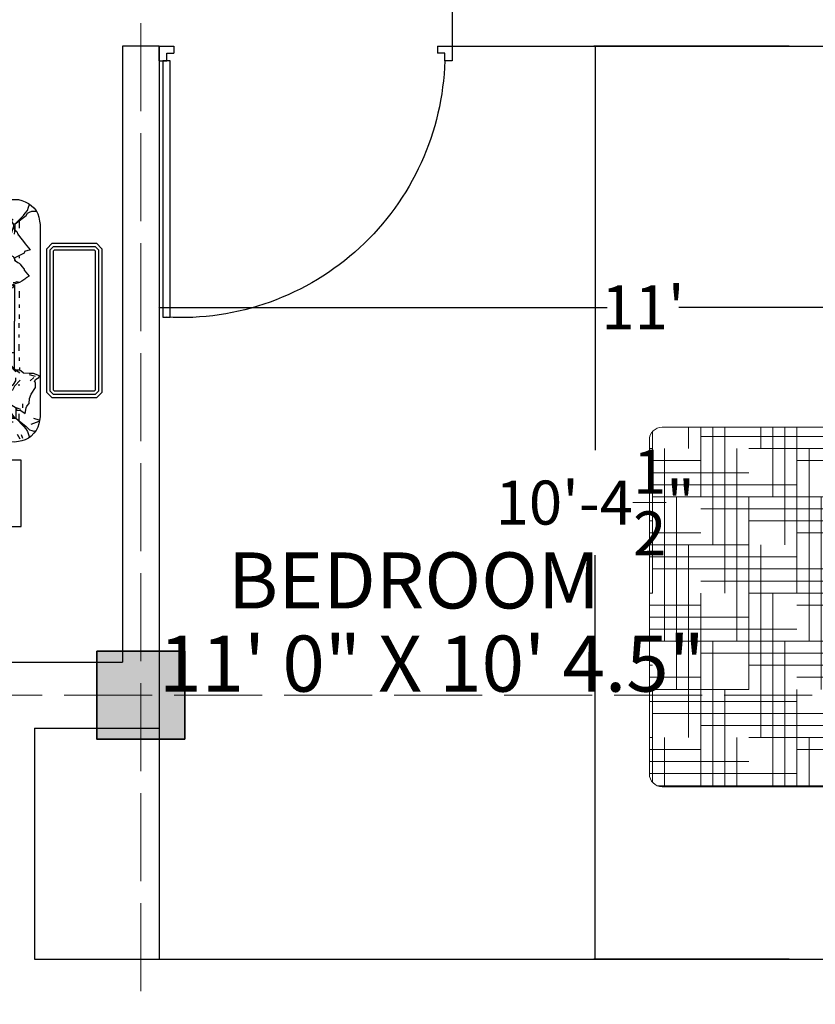
# Model space of a CAD drawing. Units: inches. Extents: x -113 to 5399, y -1393 to 3302.
# Tile 38 of 40: x 3504 to 3612, y 2903 to 3038. Entities that reach past the tile are written whole.
import ezdxf

# ---------------------------------------------------------------- set-up
doc = ezdxf.new("R2010")
doc.units = ezdxf.units.IN
doc.header["$MEASUREMENT"] = 0
doc.linetypes.add('ACAD_ISO02W100', pattern=[15, 12, -3])
doc.layers.add('24', color=7, linetype='Continuous')
for name, color, linetype, lineweight in [('A-ANNO-DIMS', 254, 'Continuous', 18), ('A-AREA-IDEN', 4, 'Continuous', 18), ('A-COLS', 7, 'Continuous', 35), ('doors', 2, 'Continuous', 25), ('furniture', 131, 'Continuous', 18), ('GRIDS', 7, 'ACAD_ISO02W100', 13), ('walls', 1, 'Continuous', 25)]:
    doc.layers.add(name, color=color, linetype=linetype, lineweight=lineweight)
doc.styles.get("Standard").update_dxf_attribs({"font": 'arial.ttf'})
doc.dimstyles.get("Standard").update_dxf_attribs({"dimtxt": 6, "dimasz": 0.18, "dimexe": 0.18, "dimexo": 0.0625, "dimgap": 0.09, "dimtad": 0, "dimtih": 1, "dimtoh": 1, "dimdec": 1, "dimzin": 0, "dimdsep": 46, "dimlunit": 4, "dimtxsty": 'Standard', "dimblk": 'ARCHTICK', "dimcen": 0.09, "dimadec": 0, "dimazin": 0, "dimtfac": 1, "dimtdec": 1, "dimtofl": 0, "dimtmove": 0, "dimatfit": 3, "dimfxl": 1, "dimtolj": 1, "dimtzin": 0, "dimarcsym": 0})

# ---------------------------------------------------------------- blocks, each defined once
blk = doc.blocks.new('*X4')
at = {"color": 0}
for p, q in [((4.3594, 18.5625), (4.3594, 18.6457)), ((4.5, 18), (4.5, 18.6457)), ((4.5469, 18.1875), (4.5469, 18.6457)), ((4.5938, 18.375), (4.5938, 18.6457)), ((4.6406, 18.5625), (4.6406, 18.6457)), ((4.7812, 18), (4.7812, 18.6457)), ((4.8281, 18.1875), (4.8281, 18.6457)), ((4.875, 18.375), (4.875, 18.6457)), ((4.9219, 18.5625), (4.9219, 18.6457)), ((5.0625, 18), (5.0625, 18.6457)), ((5.1094, 18.1875), (5.1094, 18.6457)), ((5.1562, 18.375), (5.1562, 18.6457)), ((5.2031, 18.5625), (5.2031, 18.6457)), ((5.3438, 18), (5.3438, 18.6457)), ((5.3906, 18.1875), (5.3906, 18.6457)), ((5.4375, 18.375), (5.4375, 18.6457)), ((5.4844, 18.5625), (5.4844, 18.6457)), ((4.6875, 18.6094), (5.4375, 18.6094)), ((5.625, 18), (5.625, 18.6287)), ((4.4531, 17.8169), (4.4531, 18.5625)), ((4.5, 18.5625), (5.25, 18.5625)), ((4.7344, 17.8125), (4.7344, 18.5625)), ((5.0156, 17.8125), (5.0156, 18.5625)), ((5.2969, 17.8125), (5.2969, 18.5625)), ((5.5781, 17.8125), (5.5781, 18.5625)), ((5.625, 18.5625), (5.6375, 18.5625)), ((4.3395, 18.5156), (5.0625, 18.5156)), ((5.4375, 18.5156), (5.6375, 18.5156)), ((4.3395, 18.4688), (4.875, 18.4688)), ((5.25, 18.4688), (5.6375, 18.4688)), ((4.3395, 18.4219), (4.6875, 18.4219)), ((5.0625, 18.4219), (5.6375, 18.4219)), ((4.3395, 18.375), (4.5, 18.375)), ((4.4062, 17.8169), (4.4062, 18.375)), ((4.6875, 17.8114), (4.6875, 18.375)), ((4.875, 18.375), (5.625, 18.375)), ((4.9688, 17.625), (4.9688, 18.375)), ((5.25, 17.625), (5.25, 18.375)), ((5.5312, 17.625), (5.5312, 18.375)), ((4.6875, 18.3281), (5.4375, 18.3281)), ((4.5, 18.2812), (5.25, 18.2812)), ((5.625, 18.2812), (5.6375, 18.2812)), ((4.3395, 18.2344), (5.0625, 18.2344)), ((5.4375, 18.2344), (5.6375, 18.2344)), ((4.3395, 18.1875), (4.875, 18.1875)), ((4.3594, 17.8169), (4.3594, 18.1875)), ((4.6406, 17.8169), (4.6406, 18.1875)), ((4.9219, 17.4375), (4.9219, 18.1875)), ((5.2031, 17.4375), (5.2031, 18.1875)), ((5.25, 18.1875), (5.6375, 18.1875)), ((5.4844, 17.4375), (5.4844, 18.1875)), ((4.3395, 18.1406), (4.6875, 18.1406)), ((5.0625, 18.1406), (5.6375, 18.1406)), ((4.3395, 18.0938), (4.5, 18.0938)), ((4.875, 18.0938), (5.625, 18.0938)), ((4.6875, 18.0469), (5.4375, 18.0469)), ((4.5, 18), (5.25, 18)), ((4.5938, 17.8169), (4.5938, 18)), ((4.875, 17.25), (4.875, 18)), ((5.1562, 17.25), (5.1562, 18)), ((5.4375, 17.25), (5.4375, 18)), ((5.625, 18), (5.6375, 18)), ((4.3395, 17.9531), (5.0625, 17.9531)), ((5.4375, 17.9531), (5.6375, 17.9531)), ((4.3395, 17.9062), (4.875, 17.9062)), ((5.25, 17.9062), (5.6375, 17.9062)), ((4.3395, 17.8594), (4.6875, 17.8594)), ((5.0625, 17.8594), (5.6375, 17.8594)), ((4.8281, 17.2457), (4.8281, 17.8125)), ((4.875, 17.8125), (5.625, 17.8125)), ((5.1094, 17.2457), (5.1094, 17.8125)), ((5.3906, 17.2457), (5.3906, 17.8125)), ((4.7421, 17.7656), (5.4375, 17.7656)), ((4.7548, 17.7188), (5.25, 17.7188)), ((5.625, 17.7188), (5.6375, 17.7188)), ((4.7548, 17.6719), (5.0625, 17.6719)), ((5.4375, 17.6719), (5.6375, 17.6719)), ((4.7548, 17.625), (4.875, 17.625)), ((4.7812, 17.2457), (4.7812, 17.625)), ((5.0625, 17.2457), (5.0625, 17.625)), ((5.25, 17.625), (5.6375, 17.625)), ((5.3438, 17.2457), (5.3438, 17.625)), ((5.625, 17.2627), (5.625, 17.625)), ((5.0625, 17.5781), (5.6375, 17.5781)), ((4.875, 17.5312), (5.625, 17.5312)), ((4.7548, 17.4844), (5.4375, 17.4844)), ((4.7548, 17.4375), (5.25, 17.4375)), ((5.0156, 17.2457), (5.0156, 17.4375)), ((5.2969, 17.2457), (5.2969, 17.4375)), ((5.5781, 17.2457), (5.5781, 17.4375)), ((5.625, 17.4375), (5.6375, 17.4375)), ((4.7548, 17.3906), (5.0625, 17.3906)), ((5.4375, 17.3906), (5.6375, 17.3906)), ((4.7548, 17.3438), (4.875, 17.3438)), ((5.25, 17.3438), (5.6375, 17.3438)), ((5.0625, 17.2969), (5.6375, 17.2969)), ((4.875, 17.25), (5.6077, 17.25)), ((4.9688, 17.2457), (4.9688, 17.25)), ((5.25, 17.2457), (5.25, 17.25)), ((5.5312, 17.2457), (5.5312, 17.25))]:
    blk.add_line(p, q, dxfattribs=at)
blk = doc.blocks.new('MAT-P01')
for p, q in [((0.0087, 0.8464), (0.2471, 0.8464)), ((0.3737, 0.8464), (1.6737, 0.8464)), ((1.7922, 0.8464), (2.0306, 0.8464)), ((-0.0213, 0.8164), (-0.0213, 0.5605)), ((0.2771, 0.8164), (0.2771, 0.5605)), ((0.3437, 0.8164), (0.3437, -0.0316)), ((1.7037, 0.8164), (1.7037, 0.5005)), ((1.7622, 0.8164), (1.7622, 0.5605)), ((2.0606, 0.8164), (2.0606, 0.5605)), ((0.0087, 0.5305), (0.2471, 0.5305)), ((0.9879, 0.5005), (1.0693, 0.5005)), ((1.6393, 0.5005), (1.7237, 0.5005)), ((1.7237, 0.5005), (1.7237, -0.8836)), ((1.7922, 0.5305), (2.0306, 0.5305)), ((0.8146, 0.423), (0.3237, -0.0509)), ((0.8949, 0.4293), (0.8949, 0.0491)), ((0.8949, 0.3643), (1.7237, 0.3643)), ((0.8949, 0.3643), (0.8949, 0.0491)), ((0.8949, 0.3643), (1.7237, 0.3643)), ((1.7237, 0.3643), (1.7237, -0.8836)), ((0.3237, -0.0509), (0.7949, -0.0509)), ((0.3237, -0.0509), (0.3237, -0.8836)), ((0.3737, -0.9336), (1.6737, -0.9336))]:
    blk.add_line(p, q)
for centre, radius, start, end in [((0.0087, 0.8164), 0.03, 90, 180), ((0.2471, 0.8164), 0.03, 0, 90), ((0.3737, 0.8164), 0.03, 90, 180), ((1.6737, 0.8164), 0.03, 0, 90), ((1.7922, 0.8164), 0.03, 90, 180), ((2.0306, 0.8164), 0.03, 0, 90), ((1.2251, 0.6034), 0.8138, 168.373, 191.627), ((0.7029, -1.1436), 1.9306, 81.8162, 98.1838), ((0.1806, 0.6034), 0.8138, 348.373, 11.627), ((1.8766, 0.6034), 0.8138, 168.373, 191.627), ((1.3543, -1.1436), 1.9306, 81.8162, 98.1838), ((0.8321, 0.6034), 0.8138, 348.373, 11.627), ((0.0087, 0.5605), 0.03, 180, 270), ((0.2471, 0.5605), 0.03, 270, 0), ((1.7922, 0.5605), 0.03, 180, 270), ((2.0306, 0.5605), 0.03, 270, 0), ((0.7029, 2.3504), 1.9306, 261.8162, 278.1838), ((1.3543, 2.3504), 1.9306, 261.8162, 278.1838), ((0.7949, 0.0491), 0.1, 270, 0), ((0.3737, -0.8836), 0.05, 180, 270), ((1.6737, -0.8836), 0.05, 270, 0)]:
    blk.add_arc(centre, radius, start, end)
at = {"rotation": 270}
blk.add_blockref('*X4', (-16.9221, 4.7038), dxfattribs=at)
blk = doc.blocks.new('DL13712')
at = {"layer": '24'}
for p, q in [((33, 28.5), (-34, 28.5)), ((33.5, -29.5), (-10, -29.5))]:
    blk.add_line(p, q, dxfattribs=at)
blk = doc.blocks.new('DL13976')
at = {"layer": '24'}
for p, q in [((-10.5, 16.5), (-7, 18.5)), ((-7, 18.5), (-3.5, 19.5)), ((-3.5, 19.5), (0.5, 20)), ((0.5, 20), (4.5, 19.5)), ((4.5, 19.5), (8, 18.5)), ((8, 18.5), (11.5, 16.5)), ((-18, 7.5), (-16, 11)), ((-16, 11), (-13.5, 14)), ((-13.5, 14), (-10.5, 16.5)), ((-4.5, 8), (-2.5, 9)), ((-2.5, 9), (0, 9.5)), ((0, 9.5), (2.5, 9.5)), ((0.5, -9.5), (0.5, 9.5)), ((2.5, 9.5), (5, 8.5)), ((11.5, 16.5), (14.5, 14)), ((14.5, 14), (17, 11)), ((17, 11), (19, 7.5)), ((-19.5, 0), (-19, 4)), ((-19, -4), (-19.5, 0)), ((-19, 4), (-18, 7.5)), ((-9, 2), (-8, 4.5)), ((-9, -0.5), (-9, 2)), ((-9, 0), (10, 0)), ((-8, 4.5), (-6.5, 6.5)), ((-6.5, 6.5), (-4.5, 8)), ((-5.5, 0), (6.5, 0)), ((0.5, -6), (0.5, 6)), ((5, 8.5), (7, 7)), ((7, 7), (8.5, 5)), ((8.5, 5), (9.5, 3)), ((9.5, 3), (10, 0.5)), ((10, 0.5), (10, -2)), ((19, 7.5), (20, 4)), ((20, 4), (20.5, 0)), ((20.5, 0), (20, -4)), ((-18, -7.5), (-19, -4)), ((-16, -11), (-18, -7.5)), ((-8.5, -3), (-9, -0.5)), ((-7.5, -5), (-8.5, -3)), ((-6, -7), (-7.5, -5)), ((-4, -8.5), (-6, -7)), ((-1.5, -9.5), (-4, -8.5)), ((5.5, -8), (3.5, -9)), ((7.5, -6.5), (5.5, -8)), ((9, -4.5), (7.5, -6.5)), ((10, -2), (9, -4.5)), ((19, -7.5), (17, -11)), ((20, -4), (19, -7.5)), ((-13.5, -14), (-16, -11)), ((-10.5, -16.5), (-13.5, -14)), ((-7, -18.5), (-10.5, -16.5)), ((1, -9.5), (-1.5, -9.5)), ((3.5, -9), (1, -9.5)), ((11.5, -16.5), (8, -18.5)), ((14.5, -14), (11.5, -16.5)), ((17, -11), (14.5, -14)), ((-3.5, -19.5), (-7, -18.5)), ((0.5, -20), (-3.5, -19.5)), ((4.5, -19.5), (0.5, -20)), ((8, -18.5), (4.5, -19.5))]:
    blk.add_line(p, q, dxfattribs=at)
blk = doc.blocks.new('DL13329')
at = {"layer": '24'}
for p, q in [((0, 0), (0, -60)), ((60, 0), (0, 0)), ((60, -60), (60, 0)), ((0, -60), (60, -60))]:
    blk.add_line(p, q, dxfattribs=at)
blk = doc.blocks.new('DL13303')
at = {"layer": '24'}
for p, q in [((-70, 20), (-65, 25)), ((-70, -20), (-70, 20)), ((-67, 19), (-64, 22)), ((-67, -19), (-67, 19)), ((-65, 25), (65, 25)), ((-64, 22), (64, 22)), ((-64, 18), (-63, 19)), ((-64, -18), (-64, 18)), ((-63, 19), (63, 19)), ((63, 19), (64, 18)), ((64, 22), (67, 19)), ((64, 18), (64, -18)), ((65, 25), (70, 20)), ((67, 19), (67, -19)), ((70, 20), (70, -20)), ((-65, -25), (-70, -20)), ((-64, -22), (-67, -19)), ((65, -25), (-65, -25)), ((-63, -19), (-64, -18)), ((64, -22), (-64, -22)), ((63, -19), (-63, -19)), ((64, -18), (63, -19)), ((67, -19), (64, -22)), ((70, -20), (65, -25))]:
    blk.add_line(p, q, dxfattribs=at)
blk = doc.blocks.new('DL12701')
at = {"layer": '24'}
for p, q in [((-93.5, 44.5), (-90, 45)), ((-90, 45), (-87, 45.5)), ((-87, 45.5), (0, 45.5)), ((0, 45.5), (87, 45.5)), ((50, 45), (48, 39.5)), ((51.5, 44.5), (50, 45)), ((87, 45.5), (90.5, 45)), ((90.5, 45), (93.5, 44.5)), ((-106, 35), (-104, 37.5)), ((-102.5, 35), (-105, 36)), ((-104, 37.5), (-102, 40)), ((-102, 40), (-99.5, 42)), ((-99.5, 42), (-96.5, 43.5)), ((-99, 40), (-99, 42)), ((-99, 38), (-99, 40)), ((-98, 36), (-99, 38)), ((-97, 34), (-98, 36)), ((-96.5, 43.5), (-93.5, 44.5)), ((-67.5, 33.5), (-64, 36.5)), ((-64, 36.5), (-62.5, 31.5)), ((48, 39.5), (48, 35.5)), ((50.5, 41.5), (49, 36)), ((53.5, 41.5), (51.5, 44.5)), ((51.5, 40), (54.5, 36.5)), ((55.5, 40.5), (53.5, 41.5)), ((56, 41.5), (55.5, 40.5)), ((60.5, 41.5), (56, 41.5)), ((66.5, 37.5), (60.5, 41.5)), ((70.5, 36), (66.5, 37.5)), ((75, 35.5), (70.5, 36)), ((88.5, 39.5), (90, 44.5)), ((91.5, 44.5), (94, 37)), ((93.5, 44.5), (96.5, 43.5)), ((96.5, 43.5), (99.5, 42)), ((97.5, 34.5), (99, 36)), ((99, 36), (99.5, 38)), ((99.5, 42), (102, 40)), ((100, 40), (99.5, 42)), ((99.5, 38), (100, 40)), ((102, 40), (104.5, 37.5)), ((103, 35), (106, 36)), ((104.5, 37.5), (106.5, 35)), ((-109.5, 26), (-108.5, 29)), ((-108.5, 29), (-107.5, 32)), ((-107.5, 32), (-106, 35)), ((-99.5, 34), (-102.5, 35)), ((-97, 32), (-99.5, 34)), ((-95, 33), (-97, 34)), ((-95, 30.5), (-97, 32)), ((-87.5, 23), (-95, 33)), ((-87.5, 23), (-95, 30.5)), ((-78, 25.5), (-76, 27)), ((-76, 27), (-71.5, 30.5)), ((-71.5, 30.5), (-69.5, 32)), ((-69.5, 32), (-67.5, 33.5)), ((-62.5, 31.5), (-61, 31)), ((-61, 31), (-59.5, 28)), ((-59.5, 28), (-57.5, 24.5)), ((-52, 26.5), (-51, 27.5)), ((-51, 27.5), (-49, 29)), ((-49, 29), (-46.5, 31)), ((-46.5, 31), (-45.5, 31)), ((-45.5, 31), (-40, 35.5)), ((-40, 35.5), (-38.5, 33)), ((-38.5, 33), (-38, 32.5)), ((-38, 32.5), (-35.5, 29)), ((-35.5, 29), (-34.5, 27)), ((-34.5, 27), (-35, 24.5)), ((-34.5, 27), (-33.5, 24)), ((42.5, 27), (45, 27)), ((45.5, 28), (45, 27)), ((45, 27), (45, 23.5)), ((47.5, 30.5), (45.5, 28)), ((46.5, 26), (47.5, 27)), ((48, 35.5), (47.5, 30.5)), ((54, 27.5), (59.5, 22.5)), ((77.5, 33.5), (75, 35.5)), ((79, 30), (75.5, 30)), ((79, 33), (77.5, 33.5)), ((84, 32), (79, 33)), ((80.5, 28), (79, 24)), ((81, 24.5), (81.5, 28)), ((81.5, 28), (84, 32)), ((88.5, 23.5), (96, 33)), ((88.5, 23.5), (95.5, 30.5)), ((95.5, 30.5), (98, 32.5)), ((96, 33), (97.5, 34.5)), ((98, 32.5), (100.5, 34)), ((100.5, 34), (103, 35)), ((103, 28.5), (106.5, 29.5)), ((107.5, 27.5), (103, 25)), ((106.5, 35), (108, 32)), ((108, 32), (109, 29)), ((109, 29), (109.5, 26)), ((-109.5, 22.5), (-109.5, 26)), ((-109.5, -26.5), (-109.5, 22.5)), ((-95, 18.5), (-92, 19.5)), ((-95, 18), (-95, 18.5)), ((-94, 16.5), (-95, 18)), ((-92, 19.5), (-89, 20)), ((-91, 21), (-91, 19.5)), ((-89.5, 26.5), (-83.5, 26.5)), ((-89, 20), (-87.5, 21)), ((-87.5, 21), (-87.5, 23)), ((-81.5, 23), (-87.5, 23)), ((-87.5, 21), (-85, 21.5)), ((-85, 21.5), (-82, 22.5)), ((-85, 21.5), (-80.5, 20)), ((-82, 22.5), (-80.5, 24.5)), ((-82, 22.5), (-80.5, 22.5)), ((-80.5, 24.5), (-78, 25.5)), ((-80.5, 24.5), (-80.5, 23.5)), ((-80.5, 22.5), (-78, 22)), ((-80.5, 20), (-79.5, 20)), ((-77, 25.5), (-77, 25.5)), ((-60.5, 17.5), (-59, 19.5)), ((-59, 19.5), (-58.5, 19.5)), ((-58.5, 19.5), (-58, 21)), ((-58, 26.5), (-56.5, 26.5)), ((-58, 21), (-54.5, 23)), ((-57.5, 24.5), (-56.5, 22)), ((-56.5, 22.5), (-54.5, 22.5)), ((-54.5, 22.5), (-52.5, 25.5)), ((-54.5, 23), (-54.5, 22.5)), ((-54, 22.5), (-54, 22.5)), ((-52.5, 25.5), (-52, 26.5)), ((-35, 24.5), (-34.5, 23)), ((-34.5, 23), (-34, 21)), ((-33.5, 24), (-33, 22)), ((-30, 21), (-33, 22)), ((-33, 22), (-31.5, 19.5)), ((-32, 22.5), (0.5, 22.5)), ((-31.5, 19.5), (-31, 18)), ((-29.5, 19.5), (-30, 21)), ((-28.5, 16.5), (-29.5, 19.5)), ((-26.5, 26.5), (-20.5, 26.5)), ((-14.5, 26.5), (-11.5, 26.5)), ((-5.5, 26.5), (-1.5, 26.5)), ((44, 22.5), (0.5, 22.5)), ((6.5, 26.5), (2.5, 26.5)), ((15.5, 26.5), (12.5, 26.5)), ((27.5, 26.5), (21.5, 26.5)), ((33.5, 26.5), (36.5, 26.5)), ((40.5, 18.5), (38, 14.5)), ((41.5, 20), (40.5, 18.5)), ((43.5, 22), (41.5, 20)), ((43.5, 20.5), (41.5, 20)), ((45, 23.5), (43.5, 22)), ((45, 22), (43.5, 20.5)), ((45, 23.5), (46.5, 26)), ((46.5, 23.5), (45, 22)), ((54.5, 23.5), (52, 23.5)), ((58, 21.5), (54.5, 23.5)), ((59, 26.5), (57.5, 26.5)), ((59.5, 19), (58, 21.5)), ((59.5, 22.5), (63, 20.5)), ((64, 17.5), (59.5, 19)), ((63, 20.5), (64, 17.5)), ((76, 19), (79, 24)), ((76, 16), (76, 19)), ((79, 24), (81, 24.5)), ((79, 23.5), (88.5, 23.5)), ((82.5, 18.5), (88, 22.5)), ((90.5, 26.5), (84.5, 26.5)), ((85, 16), (88, 22.5)), ((88.5, 8), (88.5, 23.5)), ((92, 21), (92, 15)), ((109.5, 26), (110, 22.5)), ((110, 22.5), (109.5, -26.5)), ((-92.5, 14), (-94, 16.5)), ((-92, 13.5), (-92.5, 14)), ((-91.5, 12.5), (-92, 13.5)), ((-89.5, 11), (-91.5, 12.5)), ((-91, 9), (-91, 6)), ((-89, 9), (-89.5, 11)), ((-89, 8.5), (-89, 9)), ((-74, 14.5), (-77.5, 15)), ((-70.5, 13.5), (-74, 14.5)), ((-74, 14.5), (-71, 10)), ((-71, 10), (-68, 8.5)), ((-67.5, 10.5), (-70.5, 13.5)), ((-68, 12), (-67.5, 12.5)), ((-65, 9), (-68, 12)), ((-67.5, 12.5), (-66.5, 13.5)), ((-61.5, 5.5), (-67.5, 10.5)), ((-66.5, 13.5), (-64.5, 15.5)), ((-63, 9), (-65, 9)), ((-64.5, 15.5), (-63.5, 15.5)), ((-63.5, 15.5), (-62.5, 16.5)), ((-62, 6.5), (-63, 9)), ((-62.5, 16.5), (-60.5, 17.5)), ((-46.5, 7.5), (-42.5, 10.5)), ((-40, 9), (-43.5, 7.5)), ((-42.5, 10.5), (-40, 11.5)), ((-40, 11.5), (-37, 13.5)), ((-32.5, 11.5), (-40, 9)), ((-37, 13.5), (-36, 14.5)), ((-24.5, 13.5), (-28.5, 16.5)), ((-21, 11), (-24.5, 13.5)), ((-19, 8.5), (-22.5, 11.5)), ((-17, 8), (-21, 11)), ((38, 14), (37.5, 11)), ((37.5, 11), (43.5, 8.5)), ((38, 14.5), (38, 14)), ((64, 17.5), (66.5, 14.5)), ((70.5, 13.5), (70.5, 14.5)), ((73, 8.5), (70.5, 13.5)), ((73, 13), (72.5, 15)), ((73, 12.5), (75, 14.5)), ((73, 12.5), (73, 13)), ((73, 8.5), (73, 12.5)), ((76, 12.5), (74, 14)), ((75, 14.5), (76, 16)), ((75.5, 16), (76, 16.5)), ((80, 11), (76, 12.5)), ((80.5, 9), (79, 9)), ((80.5, 10.5), (80, 11)), ((83, 8.5), (80.5, 10.5)), ((83, 8.5), (80.5, 9)), ((92, 9), (92, 6)), ((-91, 0.5), (-91, -5.5)), ((-89, 6), (-89, 8.5)), ((-86.5, 3.5), (-89, 6)), ((-87, 3.5), (-87, -26.5)), ((-86, 3.5), (-86.5, 3.5)), ((-85.5, 0.5), (-86, 3.5)), ((-85.5, 0), (-85.5, 0.5)), ((-84.5, -2), (-85.5, 0)), ((-68, 8.5), (-66.5, 5.5)), ((-66.5, 5.5), (-66, 4)), ((-62.5, 0), (-63.5, -1)), ((-60, 6), (-62, 6.5)), ((-61, -2), (-58.5, 0.5)), ((-57.5, 3.5), (-60, 6)), ((-60, 6), (-55, 5.5)), ((-58.5, 0.5), (-55.5, 2)), ((-56.5, 3.5), (-57.5, 3.5)), ((-57.5, 3.5), (-56, 1.5)), ((-54, 3), (-56.5, 3.5)), ((-56, 1.5), (-55, 0)), ((-55, 5.5), (-54, 5)), ((-55, 0), (-52.5, -2.5)), ((-46.5, 7.5), (-50.5, 8.5)), ((-43.5, 7.5), (-46.5, 7.5)), ((-31.5, -3), (-25.5, 0)), ((-25.5, 0), (-23, 3.5)), ((-20.5, 7.5), (-25, 7)), ((-23, 5.5), (-21.5, 6)), ((-23, 3.5), (-23, 5.5)), ((-21.5, 6), (-18, 6)), ((-18, 6), (-17, 8)), ((43.5, 8.5), (44, 8)), ((44, 8), (47, 6.5)), ((47, 6.5), (49.5, 5.5)), ((49.5, 5.5), (51, 5)), ((51, 5), (52.5, 5)), ((52, -2.5), (55, 1)), ((52.5, 5), (55.5, 5)), ((55, 1), (57.5, 3)), ((55.5, 5), (55.5, 5)), ((55.5, 5), (59, 2.5)), ((59, 2.5), (60, 3.5)), ((60, 3.5), (60, 2.5)), ((60, 2.5), (63, 2)), ((63, 2), (64, 1)), ((64, 1), (66, 0.5)), ((66, 0.5), (66.5, 0)), ((66.5, 0), (69, -0.5)), ((71.5, -1), (72.5, 2.5)), ((72, 5), (73, 6.5)), ((73, 5.5), (72, -1)), ((72.5, 2.5), (72, 5)), ((73, 6.5), (73, 8.5)), ((74.5, -0.5), (76, 1.5)), ((76, 1.5), (76.5, 3)), ((84, 6.5), (81.5, 6.5)), ((85, 8), (83, 8.5)), ((85.5, 6.5), (84, 6.5)), ((88, 7.5), (85, 8)), ((88, 7.5), (85.5, 6.5)), ((90, 6.5), (88, 7.5)), ((94, 5), (90, 6.5)), ((95, 4.5), (94, 5)), ((94, -3), (97.5, 3)), ((97.5, 3), (95, 4.5)), ((-83, -4), (-84.5, -2)), ((-80.5, -6.5), (-83, -4)), ((-80.5, -7), (-80.5, -6.5)), ((-77.5, -13), (-80.5, -7)), ((-70.5, -8.5), (-73.5, -11)), ((-68.5, -7), (-70.5, -8.5)), ((-68.5, -4.5), (-67, -3)), ((-66.5, -4.5), (-68.5, -7)), ((-68.5, -7), (-68.5, -4.5)), ((-67, -3), (-66, -1)), ((-65.5, -3), (-66.5, -4.5)), ((-63.5, -1), (-65.5, -3)), ((-65.5, -3), (-62.5, -2.5)), ((-62.5, -2.5), (-61, -2)), ((-54, -0.5), (-53.5, -0.5)), ((-52.5, -2.5), (-49.5, -7.5)), ((-49.5, -7.5), (-49.5, -9)), ((-45.5, -11), (-48.5, -7.5)), ((-43, -10), (-41.5, -7)), ((-38, -9), (-35, -6.5)), ((-35, -6.5), (-31.5, -3)), ((48, -10), (51.5, -6)), ((51.5, -5.5), (52, -2.5)), ((51.5, -6), (51.5, -5.5)), ((52, -8), (55.5, -5.5)), ((69, -0.5), (70.5, -1)), ((70.5, -1), (71.5, -1)), ((72, -1), (70.5, -5)), ((70.5, -5), (72.5, -8)), ((72.5, -8), (74.5, -3.5)), ((72.5, -8), (73, -12.5)), ((74.5, -3.5), (74.5, -0.5)), ((91, -10), (92, -8.5)), ((92, -8.5), (93, -7)), ((93, -7), (93.5, -4)), ((93.5, -4), (94, -3)), ((-91, -14), (-91, -11)), ((-74.5, -11.5), (-77.5, -13)), ((-73.5, -11), (-74.5, -11.5)), ((-49.5, -9), (-47, -11.5)), ((-47, -11.5), (-45, -15.5)), ((-45, -15.5), (-42, -11.5)), ((-42, -11.5), (-41, -11)), ((-41, -11), (-38, -9)), ((52, -12), (48, -10)), ((52, -10), (56.5, -12.5)), ((55, -13), (52, -12)), ((56.5, -13), (55, -13)), ((62.5, -16), (56.5, -13)), ((64.5, -17), (62.5, -16)), ((64, -16.5), (64, -16.5)), ((66.5, -18), (64.5, -17)), ((67.5, -15.5), (68.5, -18)), ((70, -16.5), (69.5, -15.5)), ((72, -21), (70, -16.5)), ((85, -17.5), (87, -16.5)), ((85, -18), (85, -17.5)), ((87, -16.5), (88, -13)), ((87.5, -12.5), (89.5, -11)), ((88, -13), (87.5, -12.5)), ((87.5, -26.5), (87.5, -14.5)), ((89.5, -11), (91, -10)), ((92, -14), (92, -11)), ((-109.5, -28), (-109.5, -26.5)), ((-109.5, -26.5), (-109.5, -29.5)), ((-106, -26), (-104.5, -26)), ((-102.5, -26), (-100.5, -26)), ((-98.5, -26), (-96, -26)), ((-94.5, -26), (-92.5, -26)), ((-91, -26), (-91, -20)), ((-87, -26.5), (-87, -28)), ((69, -18.5), (66.5, -18)), ((68.5, -18), (69, -18.5)), ((69, -18.5), (72, -21)), ((72, -21), (73, -22.5)), ((73, -22.5), (74.5, -23.5)), ((74.5, -23.5), (76, -26)), ((76, -26), (79, -28)), ((79.5, -27.5), (80, -26)), ((80, -26), (82.5, -23.5)), ((82.5, -21.5), (83.5, -20)), ((82.5, -22.5), (82.5, -21.5)), ((82.5, -23.5), (82.5, -22.5)), ((83.5, -20), (85, -18)), ((87.5, -28), (87.5, -26.5)), ((92, -26), (92, -20)), ((95.5, -26), (93.5, -26)), ((99.5, -26), (97, -26)), ((103.5, -26), (101.5, -26)), ((107, -26), (105.5, -26)), ((110, -29.5), (109.5, -26.5)), ((109.5, -26.5), (109.5, -28)), ((-109, -29), (-109.5, -28)), ((-109.5, -29.5), (-109, -32.5)), ((-108.5, -30), (-109, -29)), ((-109, -32.5), (-108, -35)), ((-108, -31), (-108.5, -30)), ((-106.5, -31.5), (-108, -31)), ((-108, -35), (-107, -37.5)), ((-105.5, -31.5), (-106.5, -31.5)), ((-104.5, -31.5), (-105.5, -31.5)), ((-92, -31.5), (-104.5, -31.5)), ((-91, -31.5), (-92, -31.5)), ((-90, -31.5), (-91, -31.5)), ((-90.5, -27.5), (-88, -28)), ((-90.5, -28), (-90, -29)), ((-89, -30.5), (-90, -31.5)), ((-88, -30), (-89, -30.5)), ((-87.5, -29), (-88, -30)), ((-87, -28), (-87.5, -29)), ((79, -28), (79.5, -27.5)), ((87.5, -29), (87.5, -28)), ((88, -30), (87.5, -29)), ((89, -30.5), (88, -30)), ((91.5, -27.5), (89, -28)), ((90, -31.5), (89, -30.5)), ((91, -31.5), (90, -31.5)), ((91.5, -28), (91, -29)), ((92.5, -31.5), (91, -31.5)), ((104.5, -31.5), (92.5, -31.5)), ((106, -31.5), (104.5, -31.5)), ((107, -31.5), (106, -31.5)), ((108, -31), (107, -31.5)), ((107, -37.5), (108.5, -35)), ((109, -30), (108, -31)), ((108.5, -35), (109.5, -32.5)), ((109.5, -29), (109, -30)), ((109.5, -28), (109.5, -29)), ((109.5, -32.5), (110, -29.5)), ((-107, -37.5), (-105, -39.5)), ((-105, -39.5), (-102.5, -41.5)), ((-102.5, -41.5), (-100, -43)), ((-100.5, -37), (-100.5, -40.5)), ((-100, -43), (-97.5, -44)), ((-94.5, -39.5), (-98.5, -42.5)), ((-97.5, -44), (-94.5, -44.5)), ((-94.5, -44.5), (0, -44.5)), ((-67, -37), (-64.5, -40.5)), ((-45, -37.5), (-49.5, -41)), ((-27.5, -37.5), (-29.5, -42.5)), ((0, -44.5), (95, -44.5)), ((28.5, -37.5), (30.5, -42.5)), ((46, -37.5), (50.5, -41)), ((68, -37), (65.5, -40.5)), ((95, -44.5), (97.5, -44)), ((95.5, -39.5), (99.5, -42.5)), ((97.5, -44), (100.5, -43)), ((100.5, -43), (103, -41.5)), ((101.5, -37), (101.5, -40.5)), ((103, -41.5), (105, -39.5)), ((105, -39.5), (107, -37.5))]:
    blk.add_line(p, q, dxfattribs=at)
blk = doc.blocks.new('DL13707')
at = {"layer": '24'}
for p, q in [((0, -33.5), (0, 33.5)), ((-58.5, -33.5), (-58.5, 21.5)), ((58.5, -33.5), (58.5, 2))]:
    blk.add_line(p, q, dxfattribs=at)
blk = doc.blocks.new('DL13651')
at = {"layer": '24'}
for p, q in [((-50.5, 25), (-50, 27)), ((-50, 27), (-49, 28.5)), ((-49, 28.5), (-47.5, 29.5)), ((-47.5, 29.5), (-45.5, 30)), ((-45.5, 30), (44.5, 30)), ((44.5, 30), (46.5, 29.5)), ((46.5, 29.5), (48, 28.5)), ((48, 28.5), (49, 27)), ((49, 27), (49.5, 25)), ((-50.5, -25), (-50.5, 25)), ((-45.5, 24.5), (-45.5, 25)), ((-45.5, 25), (-45, 25)), ((-45.5, -24.5), (-45.5, 24.5)), ((-45, 25), (44, 25)), ((-45, 22), (44, 22)), ((-42.5, 22), (-45, 22)), ((-42.5, -24.5), (-42.5, 24.5)), ((-42.5, 24.5), (-42.5, 22)), ((41.5, 22), (41.5, 24.5)), ((41.5, 24.5), (41.5, -24.5)), ((44, 22), (41.5, 22)), ((44, 25), (44.5, 25)), ((44.5, 25), (44.5, 24.5)), ((44.5, 24.5), (44.5, -24.5)), ((49.5, 25), (49.5, -25)), ((-50, -27), (-50.5, -25)), ((-45.5, -25), (-45.5, -24.5)), ((-45, -25), (-45.5, -25)), ((44, -22), (-45, -22)), ((-45, -22), (-42.5, -22)), ((44, -25), (-45, -25)), ((-42.5, -22), (-42.5, -24.5)), ((41.5, -24.5), (41.5, -22)), ((41.5, -22), (44, -22)), ((44.5, -25), (44, -25)), ((44.5, -24.5), (44.5, -25)), ((49.5, -25), (49, -27)), ((-49, -28.5), (-50, -27)), ((-47.5, -29.5), (-49, -28.5)), ((-45.5, -30), (-47.5, -29.5)), ((44.5, -30), (-45.5, -30)), ((46.5, -29.5), (44.5, -30)), ((48, -28.5), (46.5, -29.5)), ((49, -27), (48, -28.5))]:
    blk.add_line(p, q, dxfattribs=at)
blk = doc.blocks.new('DL12263')
at = {"layer": '24'}
for p, q in [((-112.5, 44.5), (-109, 45)), ((-109, 45), (-106, 45.5)), ((-106, 45.5), (-19, 45.5)), ((-19, 45.5), (106.5, 45.5)), ((69.5, 45), (67.5, 39.5)), ((71, 44.5), (69.5, 45)), ((106.5, 45.5), (110, 45)), ((110, 45), (113, 44.5)), ((-125, 35), (-123, 37.5)), ((-121.5, 35), (-124, 36)), ((-123, 37.5), (-121, 40)), ((-121, 40), (-118.5, 42)), ((-118.5, 42), (-115.5, 43.5)), ((-118, 40), (-118, 42)), ((-118, 38), (-118, 40)), ((-117, 36), (-118, 38)), ((-116, 34), (-117, 36)), ((-115.5, 43.5), (-112.5, 44.5)), ((-86.5, 33.5), (-83, 36.5)), ((-83, 36.5), (-81.5, 31.5)), ((67.5, 39.5), (67.5, 35.5)), ((70, 41.5), (68.5, 36)), ((73, 41.5), (71, 44.5)), ((71, 40), (74, 36.5)), ((75, 40.5), (73, 41.5)), ((75.5, 41.5), (75, 40.5)), ((80, 41.5), (75.5, 41.5)), ((86, 37.5), (80, 41.5)), ((90, 36), (86, 37.5)), ((94.5, 35.5), (90, 36)), ((108, 39.5), (109.5, 44.5)), ((111, 44.5), (113.5, 37)), ((113, 44.5), (116, 43.5)), ((116, 43.5), (119, 42)), ((117, 34.5), (118.5, 36)), ((118.5, 36), (119, 38)), ((119, 42), (121.5, 40)), ((119.5, 40), (119, 42)), ((119, 38), (119.5, 40)), ((121.5, 40), (124, 37.5)), ((122.5, 35), (125.5, 36)), ((124, 37.5), (126, 35)), ((-128.5, 26), (-127.5, 29)), ((-127.5, 29), (-126.5, 32)), ((-126.5, 32), (-125, 35)), ((-118.5, 34), (-121.5, 35)), ((-116, 32), (-118.5, 34)), ((-114, 33), (-116, 34)), ((-114, 30.5), (-116, 32)), ((-106.5, 23), (-114, 33)), ((-106.5, 23), (-114, 30.5)), ((-97, 25.5), (-95, 27)), ((-95, 27), (-90.5, 30.5)), ((-90.5, 30.5), (-88.5, 32)), ((-88.5, 32), (-86.5, 33.5)), ((-81.5, 31.5), (-80, 31)), ((-80, 31), (-78.5, 28)), ((-78.5, 28), (-76.5, 24.5)), ((-71, 26.5), (-70, 27.5)), ((-70, 27.5), (-68, 29)), ((-68, 29), (-65.5, 31)), ((-65.5, 31), (-64.5, 31)), ((-64.5, 31), (-59, 35.5)), ((-59, 35.5), (-57.5, 33)), ((-57.5, 33), (-57, 32.5)), ((-57, 32.5), (-54.5, 29)), ((-54.5, 29), (-53.5, 27)), ((-53.5, 27), (-54, 24.5)), ((-53.5, 27), (-52.5, 24)), ((62, 27), (64.5, 27)), ((65, 28), (64.5, 27)), ((64.5, 27), (64.5, 23.5)), ((67, 30.5), (65, 28)), ((66, 26), (67, 27)), ((67.5, 35.5), (67, 30.5)), ((73.5, 27.5), (79, 22.5)), ((97, 33.5), (94.5, 35.5)), ((98.5, 30), (95, 30)), ((98.5, 33), (97, 33.5)), ((103.5, 32), (98.5, 33)), ((100, 28), (98.5, 24)), ((100.5, 24.5), (101, 28)), ((101, 28), (103.5, 32)), ((108, 23.5), (115.5, 33)), ((108, 23.5), (115, 30.5)), ((115, 30.5), (117.5, 32.5)), ((115.5, 33), (117, 34.5)), ((117.5, 32.5), (120, 34)), ((120, 34), (122.5, 35)), ((122.5, 28.5), (126, 29.5)), ((127, 27.5), (122.5, 25)), ((126, 35), (127.5, 32)), ((127.5, 32), (128.5, 29)), ((128.5, 29), (129, 26)), ((-128.5, 22.5), (-128.5, 26)), ((-128.5, -26.5), (-128.5, 22.5)), ((-114, 18.5), (-111, 19.5)), ((-114, 18), (-114, 18.5)), ((-113, 16.5), (-114, 18)), ((-111, 19.5), (-108, 20)), ((-110, 21), (-110, 19.5)), ((-108.5, 26.5), (-102.5, 26.5)), ((-108, 20), (-106.5, 21)), ((-106.5, 21), (-106.5, 23)), ((-100.5, 23), (-106.5, 23)), ((-106.5, 21), (-104, 21.5)), ((-104, 21.5), (-101, 22.5)), ((-104, 21.5), (-99.5, 20)), ((-101, 22.5), (-99.5, 24.5)), ((-101, 22.5), (-99.5, 22.5)), ((-99.5, 24.5), (-97, 25.5)), ((-99.5, 24.5), (-99.5, 23.5)), ((-99.5, 22.5), (-97, 22)), ((-99.5, 20), (-98.5, 20)), ((-96, 25.5), (-96, 25.5)), ((-79.5, 17.5), (-78, 19.5)), ((-78, 19.5), (-77.5, 19.5)), ((-77.5, 19.5), (-77, 21)), ((-77, 26.5), (-75.5, 26.5)), ((-77, 21), (-73.5, 23)), ((-76.5, 24.5), (-75.5, 22)), ((-75.5, 22.5), (-73.5, 22.5)), ((-73.5, 22.5), (-71.5, 25.5)), ((-73.5, 23), (-73.5, 22.5)), ((-73, 22.5), (-73, 22.5)), ((-71.5, 25.5), (-71, 26.5)), ((-54, 24.5), (-53.5, 23)), ((-53.5, 23), (-53, 21)), ((-52.5, 24), (-52, 22)), ((-49, 21), (-52, 22)), ((-52, 22), (-50.5, 19.5)), ((-51, 22.5), (-18.5, 22.5)), ((-50.5, 19.5), (-50, 18)), ((-48.5, 19.5), (-49, 21)), ((-47.5, 16.5), (-48.5, 19.5)), ((-45.5, 26.5), (-39.5, 26.5)), ((-33.5, 26.5), (-30.5, 26.5)), ((-24.5, 26.5), (-20.5, 26.5)), ((63.5, 22.5), (-18.5, 22.5)), ((-12.5, 26.5), (-16.5, 26.5)), ((35, 26.5), (-6.5, 26.5)), ((47, 26.5), (41, 26.5)), ((53, 26.5), (56, 26.5)), ((60, 18.5), (57.5, 14.5)), ((61, 20), (60, 18.5)), ((63, 22), (61, 20)), ((63, 20.5), (61, 20)), ((64.5, 23.5), (63, 22)), ((64.5, 22), (63, 20.5)), ((64.5, 23.5), (66, 26)), ((66, 23.5), (64.5, 22)), ((74, 23.5), (71.5, 23.5)), ((77.5, 21.5), (74, 23.5)), ((78.5, 26.5), (77, 26.5)), ((79, 19), (77.5, 21.5)), ((79, 22.5), (82.5, 20.5)), ((83.5, 17.5), (79, 19)), ((82.5, 20.5), (83.5, 17.5)), ((95.5, 19), (98.5, 24)), ((95.5, 16), (95.5, 19)), ((98.5, 24), (100.5, 24.5)), ((98.5, 23.5), (108, 23.5)), ((102, 18.5), (107.5, 22.5)), ((110, 26.5), (104, 26.5)), ((104.5, 16), (107.5, 22.5)), ((108, 8), (108, 23.5)), ((111.5, 21), (111.5, 15)), ((129, 26), (129.5, 22.5)), ((129.5, 22.5), (129, -26.5)), ((-111.5, 14), (-113, 16.5)), ((-111, 13.5), (-111.5, 14)), ((-110.5, 12.5), (-111, 13.5)), ((-108.5, 11), (-110.5, 12.5)), ((-110, 9), (-110, 6)), ((-108, 9), (-108.5, 11)), ((-108, 8.5), (-108, 9)), ((-93, 14.5), (-96.5, 15)), ((-89.5, 13.5), (-93, 14.5)), ((-93, 14.5), (-90, 10)), ((-90, 10), (-87, 8.5)), ((-86.5, 10.5), (-89.5, 13.5)), ((-87, 12), (-86.5, 12.5)), ((-84, 9), (-87, 12)), ((-86.5, 12.5), (-85.5, 13.5)), ((-80.5, 5.5), (-86.5, 10.5)), ((-85.5, 13.5), (-83.5, 15.5)), ((-82, 9), (-84, 9)), ((-83.5, 15.5), (-82.5, 15.5)), ((-82.5, 15.5), (-81.5, 16.5)), ((-81, 6.5), (-82, 9)), ((-81.5, 16.5), (-79.5, 17.5)), ((-65.5, 7.5), (-61.5, 10.5)), ((-59, 9), (-62.5, 7.5)), ((-61.5, 10.5), (-59, 11.5)), ((-59, 11.5), (-56, 13.5)), ((-51.5, 11.5), (-59, 9)), ((-56, 13.5), (-55, 14.5)), ((-43.5, 13.5), (-47.5, 16.5)), ((-40, 11), (-43.5, 13.5)), ((-38, 8.5), (-41.5, 11.5)), ((-36, 8), (-40, 11)), ((57.5, 14), (57, 11)), ((57, 11), (63, 8.5)), ((57.5, 14.5), (57.5, 14)), ((83.5, 17.5), (86, 14.5)), ((90, 13.5), (90, 14.5)), ((92.5, 8.5), (90, 13.5)), ((92.5, 13), (92, 15)), ((92.5, 12.5), (94.5, 14.5)), ((92.5, 12.5), (92.5, 13)), ((92.5, 8.5), (92.5, 12.5)), ((95.5, 12.5), (93.5, 14)), ((94.5, 14.5), (95.5, 16)), ((95, 16), (95.5, 16.5)), ((99.5, 11), (95.5, 12.5)), ((100, 9), (98.5, 9)), ((100, 10.5), (99.5, 11)), ((102.5, 8.5), (100, 10.5)), ((102.5, 8.5), (100, 9)), ((111.5, 9), (111.5, 6)), ((-110, 0.5), (-110, -5.5)), ((-108, 6), (-108, 8.5)), ((-105.5, 3.5), (-108, 6)), ((-106, 3.5), (-106, -26.5)), ((-105, 3.5), (-105.5, 3.5)), ((-104.5, 0.5), (-105, 3.5)), ((-104.5, 0), (-104.5, 0.5)), ((-103.5, -2), (-104.5, 0)), ((-87, 8.5), (-85.5, 5.5)), ((-85.5, 5.5), (-85, 4)), ((-81.5, 0), (-82.5, -1)), ((-79, 6), (-81, 6.5)), ((-80, -2), (-77.5, 0.5)), ((-76.5, 3.5), (-79, 6)), ((-79, 6), (-74, 5.5)), ((-77.5, 0.5), (-74.5, 2)), ((-75.5, 3.5), (-76.5, 3.5)), ((-76.5, 3.5), (-75, 1.5)), ((-73, 3), (-75.5, 3.5)), ((-75, 1.5), (-74, 0)), ((-74, 5.5), (-73, 5)), ((-74, 0), (-71.5, -2.5)), ((-65.5, 7.5), (-69.5, 8.5)), ((-62.5, 7.5), (-65.5, 7.5)), ((-50.5, -3), (-44.5, 0)), ((-44.5, 0), (-42, 3.5)), ((-39.5, 7.5), (-44, 7)), ((-42, 5.5), (-40.5, 6)), ((-42, 3.5), (-42, 5.5)), ((-40.5, 6), (-37, 6)), ((-37, 6), (-36, 8)), ((63, 8.5), (63.5, 8)), ((63.5, 8), (66.5, 6.5)), ((66.5, 6.5), (69, 5.5)), ((69, 5.5), (70.5, 5)), ((70.5, 5), (72, 5)), ((71.5, -2.5), (74.5, 1)), ((72, 5), (75, 5)), ((74.5, 1), (77, 3)), ((75, 5), (75, 5)), ((75, 5), (78.5, 2.5)), ((78.5, 2.5), (79.5, 3.5)), ((79.5, 3.5), (79.5, 2.5)), ((79.5, 2.5), (82.5, 2)), ((82.5, 2), (83.5, 1)), ((83.5, 1), (85.5, 0.5)), ((85.5, 0.5), (86, 0)), ((86, 0), (88.5, -0.5)), ((91, -1), (92, 2.5)), ((91.5, 5), (92.5, 6.5)), ((92.5, 5.5), (91.5, -1)), ((92, 2.5), (91.5, 5)), ((92.5, 6.5), (92.5, 8.5)), ((94, -0.5), (95.5, 1.5)), ((95.5, 1.5), (96, 3)), ((103.5, 6.5), (101, 6.5)), ((104.5, 8), (102.5, 8.5)), ((105, 6.5), (103.5, 6.5)), ((107.5, 7.5), (104.5, 8)), ((107.5, 7.5), (105, 6.5)), ((109.5, 6.5), (107.5, 7.5)), ((113.5, 5), (109.5, 6.5)), ((114.5, 4.5), (113.5, 5)), ((113.5, -3), (117, 3)), ((117, 3), (114.5, 4.5)), ((-102, -4), (-103.5, -2)), ((-99.5, -6.5), (-102, -4)), ((-99.5, -7), (-99.5, -6.5)), ((-96.5, -13), (-99.5, -7)), ((-89.5, -8.5), (-92.5, -11)), ((-87.5, -7), (-89.5, -8.5)), ((-87.5, -4.5), (-86, -3)), ((-85.5, -4.5), (-87.5, -7)), ((-87.5, -7), (-87.5, -4.5)), ((-86, -3), (-85, -1)), ((-84.5, -3), (-85.5, -4.5)), ((-82.5, -1), (-84.5, -3)), ((-84.5, -3), (-81.5, -2.5)), ((-81.5, -2.5), (-80, -2)), ((-73, -0.5), (-72.5, -0.5)), ((-71.5, -2.5), (-68.5, -7.5)), ((-68.5, -7.5), (-68.5, -9)), ((-64.5, -11), (-67.5, -7.5)), ((-62, -10), (-60.5, -7)), ((-57, -9), (-54, -6.5)), ((-54, -6.5), (-50.5, -3)), ((67.5, -10), (71, -6)), ((71, -5.5), (71.5, -2.5)), ((71, -6), (71, -5.5)), ((71.5, -8), (75, -5.5)), ((88.5, -0.5), (90, -1)), ((90, -1), (91, -1)), ((91.5, -1), (90, -5)), ((90, -5), (92, -8)), ((92, -8), (94, -3.5)), ((92, -8), (92.5, -12.5)), ((94, -3.5), (94, -0.5)), ((110.5, -10), (111.5, -8.5)), ((111.5, -8.5), (112.5, -7)), ((112.5, -7), (113, -4)), ((113, -4), (113.5, -3)), ((-110, -14), (-110, -11)), ((-93.5, -11.5), (-96.5, -13)), ((-92.5, -11), (-93.5, -11.5)), ((-68.5, -9), (-66, -11.5)), ((-66, -11.5), (-64, -15.5)), ((-64, -15.5), (-61, -11.5)), ((-61, -11.5), (-60, -11)), ((-60, -11), (-57, -9)), ((71.5, -12), (67.5, -10)), ((71.5, -10), (76, -12.5)), ((74.5, -13), (71.5, -12)), ((76, -13), (74.5, -13)), ((82, -16), (76, -13)), ((84, -17), (82, -16)), ((83.5, -16.5), (83.5, -16.5)), ((86, -18), (84, -17)), ((87, -15.5), (88, -18)), ((89.5, -16.5), (89, -15.5)), ((91.5, -21), (89.5, -16.5)), ((104.5, -17.5), (106.5, -16.5)), ((104.5, -18), (104.5, -17.5)), ((106.5, -16.5), (107.5, -13)), ((107, -12.5), (109, -11)), ((107.5, -13), (107, -12.5)), ((107, -26.5), (107, -14.5)), ((109, -11), (110.5, -10)), ((111.5, -14), (111.5, -11)), ((-128.5, -28), (-128.5, -26.5)), ((-128.5, -26.5), (-128.5, -29.5)), ((-125, -26), (-123.5, -26)), ((-121.5, -26), (-119.5, -26)), ((-117.5, -26), (-115, -26)), ((-113.5, -26), (-111.5, -26)), ((-110, -26), (-110, -20)), ((-106, -26.5), (-106, -28)), ((88.5, -18.5), (86, -18)), ((88, -18), (88.5, -18.5)), ((88.5, -18.5), (91.5, -21)), ((91.5, -21), (92.5, -22.5)), ((92.5, -22.5), (94, -23.5)), ((94, -23.5), (95.5, -26)), ((95.5, -26), (98.5, -28)), ((99, -27.5), (99.5, -26)), ((99.5, -26), (102, -23.5)), ((102, -21.5), (103, -20)), ((102, -22.5), (102, -21.5)), ((102, -23.5), (102, -22.5)), ((103, -20), (104.5, -18)), ((107, -28), (107, -26.5)), ((111.5, -26), (111.5, -20)), ((115, -26), (113, -26)), ((119, -26), (116.5, -26)), ((123, -26), (121, -26)), ((126.5, -26), (125, -26)), ((129.5, -29.5), (129, -26.5)), ((129, -26.5), (129, -28)), ((-128, -29), (-128.5, -28)), ((-128.5, -29.5), (-128, -32.5)), ((-127.5, -30), (-128, -29)), ((-128, -32.5), (-127, -35)), ((-127, -31), (-127.5, -30)), ((-125.5, -31.5), (-127, -31)), ((-127, -35), (-126, -37.5)), ((-124.5, -31.5), (-125.5, -31.5)), ((-123.5, -31.5), (-124.5, -31.5)), ((-111, -31.5), (-123.5, -31.5)), ((-110, -31.5), (-111, -31.5)), ((-109, -31.5), (-110, -31.5)), ((-109.5, -27.5), (-107, -28)), ((-109.5, -28), (-109, -29)), ((-108, -30.5), (-109, -31.5)), ((-107, -30), (-108, -30.5)), ((-106.5, -29), (-107, -30)), ((-106, -28), (-106.5, -29)), ((98.5, -28), (99, -27.5)), ((107, -29), (107, -28)), ((107.5, -30), (107, -29)), ((108.5, -30.5), (107.5, -30)), ((111, -27.5), (108.5, -28)), ((109.5, -31.5), (108.5, -30.5)), ((110.5, -31.5), (109.5, -31.5)), ((111, -28), (110.5, -29)), ((112, -31.5), (110.5, -31.5)), ((124, -31.5), (112, -31.5)), ((125.5, -31.5), (124, -31.5)), ((126.5, -31.5), (125.5, -31.5)), ((127.5, -31), (126.5, -31.5)), ((126.5, -37.5), (128, -35)), ((128.5, -30), (127.5, -31)), ((128, -35), (129, -32.5)), ((129, -29), (128.5, -30)), ((129, -28), (129, -29)), ((129, -32.5), (129.5, -29.5)), ((-126, -37.5), (-124, -39.5)), ((-124, -39.5), (-121.5, -41.5)), ((-121.5, -41.5), (-119, -43)), ((-119.5, -37), (-119.5, -40.5)), ((-119, -43), (-116.5, -44)), ((-113.5, -39.5), (-117.5, -42.5)), ((-116.5, -44), (-113.5, -44.5)), ((-113.5, -44.5), (-19, -44.5)), ((-86, -37), (-83.5, -40.5)), ((-64, -37.5), (-68.5, -41)), ((-46.5, -37.5), (-48.5, -42.5)), ((-19, -44.5), (114.5, -44.5)), ((48, -37.5), (50, -42.5)), ((65.5, -37.5), (70, -41)), ((87.5, -37), (85, -40.5)), ((114.5, -44.5), (117, -44)), ((115, -39.5), (119, -42.5)), ((117, -44), (120, -43)), ((120, -43), (122.5, -41.5)), ((121, -37), (121, -40.5)), ((122.5, -41.5), (124.5, -39.5)), ((124.5, -39.5), (126.5, -37.5))]:
    blk.add_line(p, q, dxfattribs=at)
blk = doc.blocks.new('U3M')
at = {"yscale": 10, "zscale": 10}
for name, p, xscale, rotation in [('DL13303', (1315, 2544), -10, 180), ('DL13976', (-270, 1769), 10, 90), ('DL13712', (1310, 1664), -10, 90), ('DL12263', (-445, 20), -10, 90), ('DL13707', (-335, 0), 10, 90), ('DL13651', (885, -25), 10, 270), ('DL12701', (1315, -1779), 10, 180), ('DL13712', (1310, -1664), 10, 90), ('DL13329', (50, -2064), 10, 180), ('DL13976', (-270, -1769), -10, 90)]:
    blk.add_blockref(name, p, dxfattribs=dict(at, xscale=xscale, rotation=rotation))
for name, p, xscale in [('DL12701', (1315, 1779), -10), ('DL13329', (50, 2064), -10), ('DL13303', (1315, -2544), 10)]:
    blk.add_blockref(name, p, dxfattribs=dict(at, xscale=xscale))
at = {"flags": 3}
for tag in ['AECLAY', 'AECGTYPE']:
    blk.add_attdef(tag, (0, 0), '', height=0.5, dxfattribs=at)
blk = doc.blocks.new('_ArchTick')
at = {"color": 0, "linetype": 'ByBlock', "const_width": 0.15}
blk.add_lwpolyline([(-0.5, -0.5), (0.5, 0.5)], dxfattribs=at)
blk = doc.blocks.new('*D148')
at = {"layer": 'A-ANNO-DIMS', "color": 0, "lineweight": -2, "transparency": 16777216}
for p, q in [((3608.48, 3034.06), (3581.85, 3034.06)), ((3582.03, 3034.06), (3582.03, 2978.97)), ((3582.03, 2909.56), (3582.03, 2964.64)), ((3608.48, 2909.56), (3581.85, 2909.56))]:
    blk.add_line(p, q, dxfattribs=at)
at = {"layer": 'Defpoints', "color": 0, "transparency": 16777216}
for p in [(3608.55, 3034.06), (3582.03, 2909.56), (3608.55, 2909.56)]:
    blk.add_point(p, dxfattribs=at)
at = {"layer": 'A-ANNO-DIMS', "color": 0, "lineweight": -2, "transparency": 16777216, "xscale": 0.18, "yscale": 0.18, "zscale": 0.18}
for p, rotation in [((3582.03, 3034.06), 90), ((3582.03, 2909.56), 270)]:
    blk.add_blockref('_ArchTick', p, dxfattribs=dict(at, rotation=rotation))
at = {"layer": 'A-ANNO-DIMS', "color": 0, "transparency": 16777216, "insert": (3582.03, 2971.81), "char_height": 6, "attachment_point": 5}
blk.add_mtext('\\A1;10\'-4{\\H1x;\\S1/2;}"', dxfattribs=at)
blk = doc.blocks.new('*D149')
at = {"layer": 'A-ANNO-DIMS', "color": 0, "lineweight": -2, "transparency": 16777216}
for p, q in [((3522.55, 2998.44), (3522.55, 2998.25)), ((3522.55, 2998.43), (3583.65, 2998.43)), ((3654.55, 2998.43), (3593.45, 2998.43)), ((3654.55, 2998.44), (3654.55, 2998.25))]:
    blk.add_line(p, q, dxfattribs=at)
at = {"layer": 'Defpoints', "color": 0, "transparency": 16777216}
for p in [(3522.55, 2998.5), (3522.55, 2998.43), (3654.55, 2998.5)]:
    blk.add_point(p, dxfattribs=at)
at = {"layer": 'A-ANNO-DIMS', "color": 0, "lineweight": -2, "transparency": 16777216, "xscale": 0.18, "yscale": 0.18, "zscale": 0.18, "rotation": 180}
blk.add_blockref('_ArchTick', (3522.55, 2998.43), dxfattribs=at)
at = {"layer": 'A-ANNO-DIMS', "color": 0, "lineweight": -2, "transparency": 16777216, "xscale": 0.18, "yscale": 0.18, "zscale": 0.18}
blk.add_blockref('_ArchTick', (3654.55, 2998.43), dxfattribs=at)
at = {"layer": 'A-ANNO-DIMS', "color": 0, "transparency": 16777216, "insert": (3588.55, 2998.43), "char_height": 6, "attachment_point": 5}
blk.add_mtext("\\A1;11'", dxfattribs=at)
blk = doc.blocks.new('COLUMN-12IN-SQUARE')
h = blk.add_hatch(color=256)
h.dxf.hatch_style = 1
h.paths.add_polyline_path([(6, 6), (-6, 6), (-6, -6), (6, -6)])
blk.add_lwpolyline([(-6, 6), (6, 6), (6, -6), (-6, -6)], close=True)
blk = doc.blocks.new('DOOR-SINGLE-36IN-PLAN')
for p, q in [((0.5, 2), (0.5, 36.98)), ((0.5, 36.98), (1.5, 36.98)), ((1.5, 36.98), (1.5, 2)), ((0, 2), (0, 0)), ((0, 2), (1.04, 2)), ((1.5, 2), (0.5, 2)), ((1.04, 2), (1.04, 0.98)), ((40, 2), (38.96, 2)), ((38.96, 2), (38.96, 0.98)), ((40, 0), (40, 2)), ((1.04, 0.98), (2, 0.98)), ((2, 0), (2, 0.98)), ((38.96, 0.98), (38, 0.98)), ((38, 0), (38, 0.98)), ((0, 0), (2, 0)), ((0, 0), (2, 0)), ((38, 0), (40, 0))]:
    blk.add_line(p, q)
blk.add_arc((2.94, 0.99), 36.04, 1.6003, 93.0893)

msp = doc.modelspace()

# ---------------------------------------------------------------- linework, layer by layer
at = {"layer": 'GRIDS'}
for p, q in [((3520.05, 3262.17), (3520.05, 2490.34)), ((3104.61, 2945.56), (3762.86, 2945.56))]:
    msp.add_line(p, q, dxfattribs=at)
at = {"layer": 'walls'}
for p, q in [((3562.55, 3063.06), (3562.55, 3034.06)), ((3517.55, 3034.06), (3517.55, 2950.06)), ((3522.55, 3034.06), (3517.55, 3034.06)), ((3522.55, 3034.06), (3522.55, 2909.56)), ((3562.55, 3034.06), (3654.55, 3034.06)), ((3421.55, 2950.06), (3517.55, 2950.06)), ((3505.55, 2941.06), (3505.55, 2909.56)), ((3505.55, 2941.06), (3522.55, 2941.06)), ((3505.55, 2909.56), (3654.55, 2909.56))]:
    msp.add_line(p, q, dxfattribs=at)

# ---------------------------------------------------------------- block references
at = {"layer": 'A-COLS'}
msp.add_blockref('COLUMN-12IN-SQUARE', (3520.05, 2945.56), dxfattribs=at)
at = {"layer": 'doors', "extrusion": (0, 0, -1), "zscale": -1, "rotation": 180}
msp.add_blockref('DOOR-SINGLE-36IN-PLAN', (-3522.55, 3034.06), dxfattribs=at)
at = {"layer": 'furniture'}
for name, p, xscale, yscale, zscale, rotation in [('U3M', (3472.65, 2976.82), 0.0150724250692195, 0.0150724250692195, 0.0150724250692195, 90), ('MAT-P01', (3622.12, 2921.72), -35.02364872074636, 35.02364872074636, 35.02364872074636, 270)]:
    msp.add_blockref(name, p, dxfattribs=dict(at, xscale=xscale, yscale=yscale, zscale=zscale, rotation=rotation))

# ---------------------------------------------------------------- texts
at = {"layer": 'A-AREA-IDEN'}
for s, height, p in [('BEDROOM', 7.647, (3531.94, 2957.37)), ('11\' 0" X 10\' 4.5"', 7.6473, (3522.55, 2946.03))]:
    msp.add_text(s, height=height, dxfattribs=at).set_placement(p)

# ---------------------------------------------------------------- dimensions: what is measured, and where the dimension line sits
at = {"layer": 'A-ANNO-DIMS'}
dim = msp.add_linear_dim(base=(3582.03, 2909.56), p1=(3608.55, 3034.06), p2=(3608.55, 2909.56), angle=90, dimstyle='Standard', override={"dimclrd": 0, "dimclre": 0, "dimclrt": 0}, dxfattribs=at)
dim.commit()
dim.dimension.update_dxf_attribs({"geometry": '*D148', "text_midpoint": (3582.03, 2971.81)})
dim = msp.add_linear_dim(base=(3522.55, 2998.43), p1=(3654.55, 2998.5), p2=(3522.55, 2998.5), dimstyle='Standard', override={"dimclrd": 0, "dimclre": 0, "dimclrt": 0}, dxfattribs=at)
dim.commit()
dim.dimension.update_dxf_attribs({"geometry": '*D149', "text_midpoint": (3588.55, 2998.43)})

doc.saveas('drawing.dxf')
